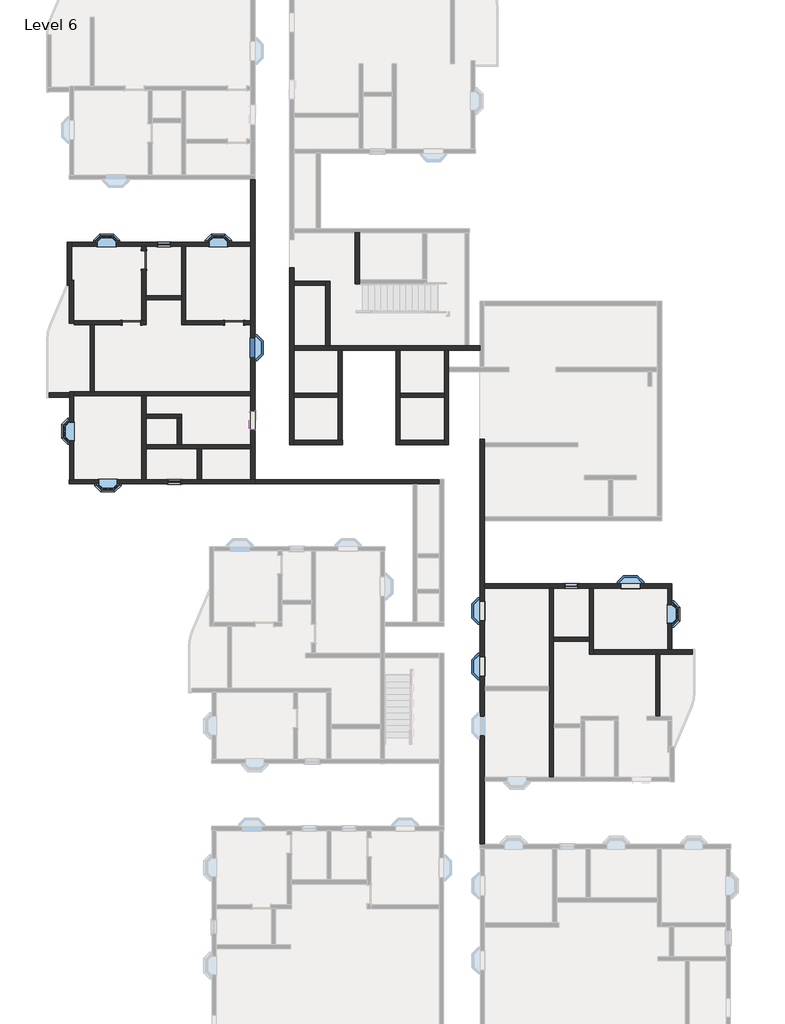
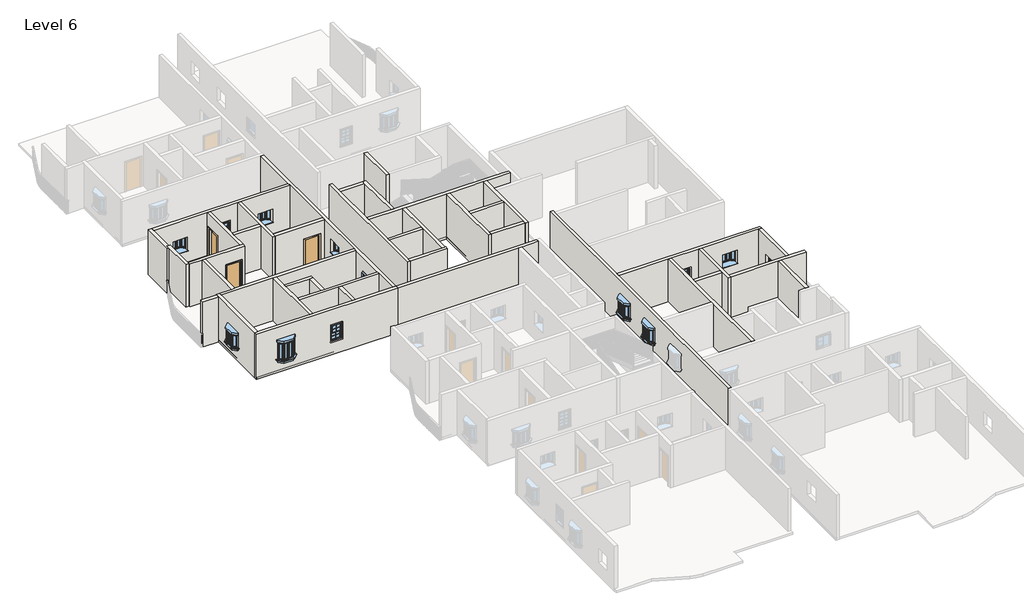
# One storey, part 3 of 14: 40 walls, 13 windows, 3 doors.
"""IFC4 building model written with IfcOpenShell, lengths in millimetres."""

from ifc_helpers import new_model, si_unit, frame, origin, place, context, project, spatial, polyline, outline, extrude, faceted_brep, transform, mapped, element, save
from components import door_54dd4da4, window_910x1210mm_154f9356, window_910x910mm_67ef725a, window_8debb0fa, windows_sgl_w_glazing_bars_910x910mm_256712d0

model = new_model("IFC4")

# Units and contexts
model_context = context("Model", 3, world=origin())
ifc_project = project(units=[si_unit("LENGTHUNIT", "METRE", prefix="MILLI")], contexts=[model_context])

# Site, building, storey
site = spatial("IfcSite", under=ifc_project)
building = spatial("IfcBuilding", under=site)
storey = spatial("IfcBuildingStorey", under=building, Name="Level 6", Elevation=15240.0)

# Doors
placement = place(None, origin())
door_shape = door_54dd4da4(model_context)
element("IfcDoor", 1, ObjectType="Single-Flush : 36\" x 84\"", at=placement, inside=storey, context=model_context, shape_type="MappedRepresentation", body=[
    mapped(door_shape, transform((-11210.3891351, 10605.7083494, 15240.0), x_axis=(1.0, 0.0, 0.0), y_axis=(0.0, 1.0, 0.0), z_axis=(0.0, 0.0, 1.0))),
])
element("IfcDoor", 2, ObjectType="Single-Flush : 36\" x 84\"", at=placement, inside=storey, context=model_context, shape_type="MappedRepresentation", body=[
    mapped(door_shape, transform((-15610.9391351, 13672.7583494, 15240.0), x_axis=(0.0, -1.0, 0.0), y_axis=(1.0, 0.0, 0.0), z_axis=(0.0, 0.0, 1.0))),
])
element("IfcDoor", 3, ObjectType="Single-Flush : 36\" x 84\"", at=placement, inside=storey, context=model_context, shape_type="MappedRepresentation", body=[
    mapped(door_shape, transform((-16220.5391351, 10605.7083494, 15240.0), x_axis=(1.0, 0.0, 0.0), y_axis=(0.0, 1.0, 0.0), z_axis=(0.0, 0.0, 1.0))),
])

# Walls
element("IfcWall", 4, ObjectType="4.5\" p", at=placement, inside=storey, context=model_context, shape_type="Brep", body=[
    faceted_brep([(-15509.3391351, 4456.3873146, 15240.0), (-13007.4391351, 4456.3873146, 15240.0), (-12804.2391351, 4456.3873146, 15240.0), (-10397.5891351, 4456.3873146, 15240.0), (-10397.5891351, 4456.3873146, 18288.0), (-12804.2391351, 4456.3873146, 18288.0), (-13007.4391351, 4456.3873146, 18288.0), (-15509.3391351, 4456.3873146, 18288.0), (-15509.3391351, 4659.5873146, 15240.0), (-15509.3391351, 4659.5873146, 18288.0), (-13985.3391351, 4659.5873146, 18288.0), (-13782.1391351, 4659.5873146, 18288.0), (-10397.5891351, 4659.5873146, 18288.0), (-10397.5891351, 4659.5873146, 15240.0), (-13782.1391351, 4659.5873146, 15240.0), (-13985.3391351, 4659.5873146, 15240.0)], [[[0, 1, 2, 3, 4, 5, 6, 7]], [[8, 9, 10, 11, 12, 13, 14, 15]], [[3, 2, 1, 0, 8, 15, 14, 13]], [[7, 6, 5, 4, 12, 11, 10, 9]], [[4, 3, 13, 12]], [[0, 7, 9, 8]]]),
])
element("IfcWall", 5, ObjectType="4.5\" p", at=placement, inside=storey, context=model_context, shape_type="SweptSolid", body=[
    extrude(outline(polyline([(-13007.4391351, 2953.9583494), (-13007.4391351, 4456.3873146), (-12804.2391351, 4456.3873146), (-12804.2391351, 2953.9583494), (-13007.4391351, 2953.9583494)])), frame((0.0, 0.0, 15240.0), z_axis=(0.0, 0.0, 1.0), x_axis=(1.0, 0.0, 0.0)), (0.0, 0.0, 1.0), 3048.0),
])
element("IfcWall", 6, ObjectType="4.5\" p", at=placement, inside=storey, context=model_context, shape_type="Brep", body=[
    faceted_brep([(-15509.3391351, 5953.2975261, 15240.0), (-13985.3391351, 5953.2975261, 15240.0), (-13782.1391351, 5953.2975261, 15240.0), (-13782.1391351, 5953.2975261, 18288.0), (-13985.3391351, 5953.2975261, 18288.0), (-15509.3391351, 5953.2975261, 18288.0), (-15509.3391351, 6156.4975261, 15240.0), (-15509.3391351, 6156.4975261, 18288.0), (-13782.1391351, 6156.4975261, 18288.0), (-13782.1391351, 6156.4975261, 15240.0)], [[[0, 1, 2, 3, 4, 5]], [[6, 7, 8, 9]], [[2, 1, 0, 6, 9]], [[5, 4, 3, 8, 7]], [[0, 5, 7, 6]], [[3, 2, 9, 8]]]),
])
element("IfcWall", 7, ObjectType="4.5\" p", at=placement, inside=storey, context=model_context, shape_type="SweptSolid", body=[
    extrude(outline(polyline([(-13985.3391351, 4659.5873146), (-13985.3391351, 5953.2975261), (-13782.1391351, 5953.2975261), (-13782.1391351, 4659.5873146), (-13985.3391351, 4659.5873146)])), frame((0.0, 0.0, 15240.0), z_axis=(0.0, 0.0, 1.0), x_axis=(1.0, 0.0, 0.0)), (0.0, 0.0, 1.0), 3048.0),
])
element("IfcWall", 8, ObjectType="4.5\" p", at=placement, inside=storey, context=model_context, shape_type="Brep", body=[
    faceted_brep([(-15712.5391351, 13215.5583494, 17373.6), (-15712.5391351, 13215.5583494, 15240.0), (-15712.5391351, 10707.3083494, 15240.0), (-15712.5391351, 10707.3083494, 18288.0), (-15712.5391351, 14333.1583494, 18288.0), (-15712.5391351, 14333.1583494, 15240.0), (-15712.5391351, 14129.9583494, 15240.0), (-15712.5391351, 14129.9583494, 17373.6), (-15509.3391351, 10707.3083494, 15240.0), (-15509.3391351, 11723.3083494, 15240.0), (-15509.3391351, 11926.5083494, 15240.0), (-15509.3391351, 13215.5583494, 15240.0), (-15509.3391351, 13215.5583494, 17373.6), (-15509.3391351, 14129.9583494, 17373.6), (-15509.3391351, 14129.9583494, 15240.0), (-15509.3391351, 14333.1583494, 15240.0), (-15509.3391351, 14333.1583494, 18288.0), (-15509.3391351, 11926.5083494, 18288.0), (-15509.3391351, 11723.3083494, 18288.0), (-15509.3391351, 10707.3083494, 18288.0)], [[[0, 1, 2, 3, 4, 5, 6, 7]], [[8, 9, 10, 11, 12, 13, 14, 15, 16, 17, 18, 19]], [[6, 5, 15, 14]], [[2, 1, 11, 10, 9, 8]], [[4, 3, 19, 18, 17, 16]], [[3, 2, 8, 19]], [[5, 4, 16, 15]], [[12, 11, 1, 0]], [[13, 12, 0, 7]], [[14, 13, 7, 6]]]),
])
element("IfcWall", 9, ObjectType="4.5\" p", at=placement, inside=storey, context=model_context, shape_type="Brep", body=[
    faceted_brep([(-13769.4391351, 14333.1583494, 15240.0), (-13769.4391351, 11926.5083494, 15240.0), (-13769.4391351, 11723.3083494, 15240.0), (-13769.4391351, 10504.1083494, 15240.0), (-13769.4391351, 10504.1083494, 18288.0), (-13769.4391351, 11723.3083494, 18288.0), (-13769.4391351, 11926.5083494, 18288.0), (-13769.4391351, 14333.1583494, 18288.0), (-13566.2391351, 14333.1583494, 15240.0), (-13566.2391351, 14333.1583494, 18288.0), (-13566.2391351, 10707.3083494, 18288.0), (-13566.2391351, 10504.1083494, 18288.0), (-13566.2391351, 10504.1083494, 15240.0), (-13566.2391351, 10707.3083494, 15240.0)], [[[0, 1, 2, 3, 4, 5, 6, 7]], [[8, 9, 10, 11, 12, 13]], [[3, 2, 1, 0, 8, 13, 12]], [[7, 6, 5, 4, 11, 10, 9]], [[0, 7, 9, 8]], [[4, 3, 12, 11]]]),
])
element("IfcWall", 10, ObjectType="4.5\" p", at=placement, inside=storey, context=model_context, shape_type="SweptSolid", body=[
    extrude(outline(polyline([(17373.6, -10753.1891351), (15240.0, -10753.1891351), (15240.0, -10397.5891351), (18288.0, -10397.5891351), (18288.0, -13566.2391351), (15240.0, -13566.2391351), (15240.0, -11667.5891351), (17373.6, -11667.5891351), (17373.6, -10753.1891351)])), frame((0.0, 10504.1083494, 0.0), z_axis=(0.0, 1.0, 0.0), x_axis=(0.0, 0.0, 1.0)), (0.0, 0.0, 1.0), 203.2),
])
element("IfcWall", 11, ObjectType="4.5\" p", at=placement, inside=storey, context=model_context, shape_type="SweptSolid", body=[
    extrude(outline(polyline([(-13769.4391351, 11723.3083494), (-15509.3391351, 11723.3083494), (-15509.3391351, 11926.5083494), (-13769.4391351, 11926.5083494), (-13769.4391351, 11723.3083494)])), frame((0.0, 0.0, 15240.0), z_axis=(0.0, 0.0, 1.0), x_axis=(1.0, 0.0, 0.0)), (0.0, 0.0, 1.0), 3048.0),
])
element("IfcWall", 12, ObjectType="4.5\" p", at=placement, inside=storey, context=model_context, shape_type="SweptSolid", body=[
    extrude(outline(polyline([(-6739.9891351, 12429.8715905), (-8289.3891351, 12429.8715905), (-8289.3891351, 12633.0715905), (-6739.9891351, 12633.0715905), (-6739.9891351, 12429.8715905)])), frame((0.0, 0.0, 15240.0), z_axis=(0.0, 0.0, 1.0), x_axis=(1.0, 0.0, 0.0)), (0.0, 0.0, 1.0), 3048.0),
])
element("IfcWall", 13, ObjectType="4.5\" p", at=placement, inside=storey, context=model_context, shape_type="SweptSolid", body=[
    extrude(outline(polyline([(-6130.3891351, 6970.2449943), (-8289.3891351, 6970.2449943), (-8289.3891351, 7173.4449943), (-6130.3891351, 7173.4449943), (-6130.3891351, 6970.2449943)])), frame((0.0, 0.0, 15240.0), z_axis=(0.0, 0.0, 1.0), x_axis=(1.0, 0.0, 0.0)), (0.0, 0.0, 1.0), 3048.0),
])
element("IfcWall", 14, ObjectType="4.5\" p", at=placement, inside=storey, context=model_context, shape_type="SweptSolid", body=[
    extrude(outline(polyline([(-948.7891351, 6970.2449943), (-3107.7891351, 6970.2449943), (-3107.7891351, 7173.4449943), (-948.7891351, 7173.4449943), (-948.7891351, 6970.2449943)])), frame((0.0, 0.0, 15240.0), z_axis=(0.0, 0.0, 1.0), x_axis=(1.0, 0.0, 0.0)), (0.0, 0.0, 1.0), 3048.0),
])
element("IfcWall", 15, ObjectType="4.5\" p", at=placement, inside=storey, context=model_context, shape_type="Brep", body=[
    faceted_brep([(-5298.5391351, 14988.9215905, 15240.0), (-5298.5391351, 12506.0715905, 15240.0), (-5298.5391351, 12506.0715905, 18288.0), (-5298.5391351, 14988.9215905, 18288.0), (-5095.3391351, 14988.9215905, 15240.0), (-5095.3391351, 14988.9215905, 18288.0), (-5095.3391351, 12709.2715905, 18288.0), (-5095.3391351, 12506.0715905, 18288.0), (-5095.3391351, 12506.0715905, 15240.0), (-5095.3391351, 12709.2715905, 15240.0)], [[[0, 1, 2, 3]], [[4, 5, 6, 7, 8, 9]], [[1, 0, 4, 9, 8]], [[3, 2, 7, 6, 5]], [[0, 3, 5, 4]], [[2, 1, 8, 7]]]),
])
element("IfcWall", 16, ObjectType="4.5\" p", at=placement, inside=storey, context=model_context, shape_type="SweptSolid", body=[
    extrude(outline(polyline([(-948.7891351, 4665.1949943), (-3107.7891351, 4665.1949943), (-3107.7891351, 4868.3949943), (-948.7891351, 4868.3949943), (-948.7891351, 4665.1949943)])), frame((0.0, 0.0, 15240.0), z_axis=(0.0, 0.0, 1.0), x_axis=(1.0, 0.0, 0.0)), (0.0, 0.0, 1.0), 3048.0),
])
element("IfcWall", 17, ObjectType="4.5\" p", at=placement, inside=storey, context=model_context, shape_type="Brep", body=[
    faceted_brep([(4184.4880523, -2336.4042694, 15240.0), (4184.4880523, -7130.6542694, 15240.0), (4184.4880523, -7333.8542694, 15240.0), (4184.4880523, -11556.6042694, 15240.0), (4184.4880523, -11556.6042694, 18288.0), (4184.4880523, -7333.8542694, 18288.0), (4184.4880523, -7130.6542694, 18288.0), (4184.4880523, -2336.4042694, 18288.0), (4387.6880523, -2336.4042694, 15240.0), (4387.6880523, -2336.4042694, 18288.0), (4387.6880523, -4736.7042694, 18288.0), (4387.6880523, -4939.9042694, 18288.0), (4387.6880523, -8959.4542694, 18288.0), (4387.6880523, -9162.6542694, 18288.0), (4387.6880523, -11556.6042694, 18288.0), (4387.6880523, -11556.6042694, 15240.0), (4387.6880523, -9162.6542694, 15240.0), (4387.6880523, -8959.4542694, 15240.0), (4387.6880523, -4939.9042694, 15240.0), (4387.6880523, -4736.7042694, 15240.0)], [[[0, 1, 2, 3, 4, 5, 6, 7]], [[8, 9, 10, 11, 12, 13, 14, 15, 16, 17, 18, 19]], [[3, 2, 1, 0, 8, 19, 18, 17, 16, 15]], [[7, 6, 5, 4, 14, 13, 12, 11, 10, 9]], [[4, 3, 15, 14]], [[0, 7, 9, 8]]]),
])
element("IfcWall", 18, ObjectType="4.5\" p", at=placement, inside=storey, context=model_context, shape_type="Brep", body=[
    faceted_brep([(803.8108649, 4915.2957306, 15240.0), (803.8108649, -14845.9042694, 15240.0), (803.8108649, -14845.9042694, 18288.0), (803.8108649, 4915.2957306, 18288.0), (803.8108649, -9516.0542694, 17350.0), (803.8108649, -9516.0542694, 16440.0), (803.8108649, -8606.0542694, 16440.0), (803.8108649, -8606.0542694, 17350.0), (803.8108649, -3909.0042694, 17350.0), (803.8108649, -3909.0042694, 16440.0), (803.8108649, -2999.0042694, 16440.0), (803.8108649, -2999.0042694, 17350.0), (803.8108649, -6620.4542694, 17350.0), (803.8108649, -6620.4542694, 16440.0), (803.8108649, -5710.4542694, 16440.0), (803.8108649, -5710.4542694, 17350.0), (1007.0108649, 4915.2957306, 15240.0), (1007.0108649, 4915.2957306, 18288.0), (1007.0108649, 4754.0949943, 18288.0), (1007.0108649, 4550.8949943, 18288.0), (1007.0108649, 1143.3957306, 18288.0), (1007.0108649, 940.1957306, 18288.0), (1007.0108649, -2133.2042694, 18288.0), (1007.0108649, -2336.4042694, 18288.0), (1007.0108649, -7130.6542694, 18288.0), (1007.0108649, -7333.8542694, 18288.0), (1007.0108649, -11556.6042694, 18288.0), (1007.0108649, -11759.8042694, 18288.0), (1007.0108649, -14845.9042694, 18288.0), (1007.0108649, -14845.9042694, 15240.0), (1007.0108649, -11759.8042694, 15240.0), (1007.0108649, -11556.6042694, 15240.0), (1007.0108649, -7333.8542694, 15240.0), (1007.0108649, -7130.6542694, 15240.0), (1007.0108649, -2336.4042694, 15240.0), (1007.0108649, -2133.2042694, 15240.0), (1007.0108649, 940.1957306, 15240.0), (1007.0108649, 1143.3957306, 15240.0), (1007.0108649, 4550.8949943, 15240.0), (1007.0108649, 4754.0949943, 15240.0), (1007.0108649, -9516.0542694, 17350.0), (1007.0108649, -8606.0542694, 17350.0), (1007.0108649, -8606.0542694, 16440.0), (1007.0108649, -9516.0542694, 16440.0), (1007.0108649, -3909.0042694, 17350.0), (1007.0108649, -2999.0042694, 17350.0), (1007.0108649, -2999.0042694, 16440.0), (1007.0108649, -3909.0042694, 16440.0), (1007.0108649, -6620.4542694, 17350.0), (1007.0108649, -5710.4542694, 17350.0), (1007.0108649, -5710.4542694, 16440.0), (1007.0108649, -6620.4542694, 16440.0)], [[[0, 1, 2, 3], [4, 5, 6, 7], [8, 9, 10, 11], [12, 13, 14, 15]], [[16, 17, 18, 19, 20, 21, 22, 23, 24, 25, 26, 27, 28, 29, 30, 31, 32, 33, 34, 35, 36, 37, 38, 39], [40, 41, 42, 43], [44, 45, 46, 47], [48, 49, 50, 51]], [[1, 0, 16, 39, 38, 37, 36, 35, 34, 33, 32, 31, 30, 29]], [[3, 2, 28, 27, 26, 25, 24, 23, 22, 21, 20, 19, 18, 17]], [[0, 3, 17, 16]], [[2, 1, 29, 28]], [[5, 4, 40, 43]], [[6, 5, 43, 42]], [[7, 6, 42, 41]], [[4, 7, 41, 40]], [[9, 8, 44, 47]], [[10, 9, 47, 46]], [[11, 10, 46, 45]], [[8, 11, 45, 44]], [[13, 12, 48, 51]], [[14, 13, 51, 50]], [[15, 14, 50, 49]], [[12, 15, 49, 48]]]),
])
element("IfcWall", 19, ObjectType="4.5\" p", at=placement, inside=storey, context=model_context, shape_type="SweptSolid", body=[
    extrude(outline(polyline([(6127.5880523, -4939.9042694), (4387.6880523, -4939.9042694), (4387.6880523, -4736.7042694), (6127.5880523, -4736.7042694), (6127.5880523, -4939.9042694)])), frame((0.0, 0.0, 15240.0), z_axis=(0.0, 0.0, 1.0), x_axis=(1.0, 0.0, 0.0)), (0.0, 0.0, 1.0), 3048.0),
])
element("IfcWall", 20, ObjectType="4.5\" p", at=placement, inside=storey, context=model_context, shape_type="Brep", body=[
    faceted_brep([(6127.5880523, -2336.4042694, 15240.0), (6127.5880523, -4736.7042694, 15240.0), (6127.5880523, -4939.9042694, 15240.0), (6127.5880523, -5555.8542694, 15240.0), (6127.5880523, -5555.8542694, 18288.0), (6127.5880523, -4939.9042694, 18288.0), (6127.5880523, -4736.7042694, 18288.0), (6127.5880523, -2336.4042694, 18288.0), (6330.7880523, -2336.4042694, 15240.0), (6330.7880523, -2336.4042694, 18288.0), (6330.7880523, -5352.6542694, 18288.0), (6330.7880523, -5555.8542694, 18288.0), (6330.7880523, -5555.8542694, 15240.0), (6330.7880523, -5352.6542694, 15240.0)], [[[0, 1, 2, 3, 4, 5, 6, 7]], [[8, 9, 10, 11, 12, 13]], [[3, 2, 1, 0, 8, 13, 12]], [[7, 6, 5, 4, 11, 10, 9]], [[0, 7, 9, 8]], [[4, 3, 12, 11]]]),
])
element("IfcWall", 21, ObjectType="4.5\" p", at=placement, inside=storey, context=model_context, shape_type="Brep", body=[
    faceted_brep([(6330.7880523, -5555.8542694, 15240.0), (9371.2322031, -5555.8542694, 15240.0), (9574.4322031, -5555.8542694, 15240.0), (11163.1380523, -5555.8542694, 15240.0), (11163.1380523, -5555.8542694, 18288.0), (9574.4322031, -5555.8542694, 18288.0), (9371.2322031, -5555.8542694, 18288.0), (6330.7880523, -5555.8542694, 18288.0), (6330.7880523, -5352.6542694, 15240.0), (6330.7880523, -5352.6542694, 18288.0), (9956.6380523, -5352.6542694, 18288.0), (10159.8380523, -5352.6542694, 18288.0), (11163.1380523, -5352.6542694, 18288.0), (11163.1380523, -5352.6542694, 15240.0), (10159.8380523, -5352.6542694, 15240.0), (9956.6380523, -5352.6542694, 15240.0)], [[[0, 1, 2, 3, 4, 5, 6, 7]], [[8, 9, 10, 11, 12, 13, 14, 15]], [[3, 2, 1, 0, 8, 15, 14, 13]], [[4, 3, 13, 12]], [[7, 6, 5, 4, 12, 11, 10, 9]], [[0, 7, 9, 8]]]),
])
element("IfcWall", 22, ObjectType="4.5\" p", at=placement, inside=storey, context=model_context, shape_type="SweptSolid", body=[
    extrude(outline(polyline([(9371.2322031, -8578.4542694), (9371.2322031, -5555.8542694), (9574.4322031, -5555.8542694), (9574.4322031, -8578.4542694), (9371.2322031, -8578.4542694)])), frame((0.0, 0.0, 15240.0), z_axis=(0.0, 0.0, 1.0), x_axis=(1.0, 0.0, 0.0)), (0.0, 0.0, 1.0), 3048.0),
])
element("IfcWall", 23, ObjectType="9\"", at=placement, inside=storey, context=model_context, shape_type="Brep", body=[
    faceted_brep([(-10181.6891351, 2953.9583494, 15240.0), (-10194.3891351, 2953.9583494, 15240.0), (-10397.5891351, 2953.9583494, 15240.0), (-12804.2391351, 2953.9583494, 15240.0), (-13007.4391351, 2953.9583494, 15240.0), (-15509.3391351, 2953.9583494, 15240.0), (-15712.5391351, 2953.9583494, 15240.0), (-19033.5891351, 2953.9583494, 15240.0), (-19236.7891351, 2953.9583494, 15240.0), (-19249.4891351, 2953.9583494, 15240.0), (-19249.4891351, 2953.9583494, 18288.0), (-19236.7891351, 2953.9583494, 18288.0), (-19033.5891351, 2953.9583494, 18288.0), (-15712.5391351, 2953.9583494, 18288.0), (-15509.3391351, 2953.9583494, 18288.0), (-13007.4391351, 2953.9583494, 18288.0), (-12804.2391351, 2953.9583494, 18288.0), (-10397.5891351, 2953.9583494, 18288.0), (-10194.3891351, 2953.9583494, 18288.0), (-10181.6891351, 2953.9583494, 18288.0), (-13794.8391351, 2953.9583494, 17221.2), (-14455.2391351, 2953.9583494, 17221.2), (-14455.2391351, 2953.9583494, 16154.4), (-13794.8391351, 2953.9583494, 16154.4), (-16918.0641351, 2953.9583494, 17350.0), (-17828.0641351, 2953.9583494, 17350.0), (-17828.0641351, 2953.9583494, 16140.0), (-16918.0641351, 2953.9583494, 16140.0), (-10181.6891351, 2750.7583494, 15240.0), (-10181.6891351, 2750.7583494, 18288.0), (-19249.4891351, 2750.7583494, 18288.0), (-19249.4891351, 2750.7583494, 15240.0), (-13794.8391351, 2750.7583494, 17221.2), (-13794.8391351, 2750.7583494, 16154.4), (-14455.2391351, 2750.7583494, 16154.4), (-14455.2391351, 2750.7583494, 17221.2), (-16918.0641351, 2750.7583494, 17350.0), (-16918.0641351, 2750.7583494, 16140.0), (-17828.0641351, 2750.7583494, 16140.0), (-17828.0641351, 2750.7583494, 17350.0)], [[[0, 1, 2, 3, 4, 5, 6, 7, 8, 9, 10, 11, 12, 13, 14, 15, 16, 17, 18, 19], [20, 21, 22, 23], [24, 25, 26, 27]], [[28, 29, 30, 31], [32, 33, 34, 35], [36, 37, 38, 39]], [[9, 8, 7, 6, 5, 4, 3, 2, 1, 0, 28, 31]], [[10, 9, 31, 30]], [[19, 18, 17, 16, 15, 14, 13, 12, 11, 10, 30, 29]], [[0, 19, 29, 28]], [[33, 32, 20, 23]], [[34, 33, 23, 22]], [[35, 34, 22, 21]], [[32, 35, 21, 20]], [[37, 36, 24, 27]], [[38, 37, 27, 26]], [[39, 38, 26, 25]], [[36, 39, 25, 24]]]),
])
element("IfcWall", 24, ObjectType="9\"", at=placement, inside=storey, context=model_context, shape_type="Brep", body=[
    faceted_brep([(-19033.5891351, 2953.9583494, 15240.0), (-19033.5891351, 7037.0083494, 15240.0), (-19033.5891351, 7240.2083494, 15240.0), (-19033.5891351, 7240.2083494, 18288.0), (-19033.5891351, 7037.0083494, 18288.0), (-19033.5891351, 2953.9583494, 18288.0), (-19033.5891351, 4854.8083494, 17064.4), (-19033.5891351, 5764.8083494, 17064.4), (-19033.5891351, 5764.8083494, 16154.4), (-19033.5891351, 4854.8083494, 16154.4), (-19236.7891351, 2953.9583494, 15240.0), (-19236.7891351, 2953.9583494, 18288.0), (-19236.7891351, 7240.2083494, 18288.0), (-19236.7891351, 7240.2083494, 15240.0), (-19236.7891351, 4854.8083494, 17064.4), (-19236.7891351, 4854.8083494, 16154.4), (-19236.7891351, 5764.8083494, 16154.4), (-19236.7891351, 5764.8083494, 17064.4)], [[[0, 1, 2, 3, 4, 5], [6, 7, 8, 9]], [[10, 11, 12, 13], [14, 15, 16, 17]], [[2, 1, 0, 10, 13]], [[5, 4, 3, 12, 11]], [[0, 5, 11, 10]], [[3, 2, 13, 12]], [[15, 14, 6, 9]], [[16, 15, 9, 8]], [[17, 16, 8, 7]], [[14, 17, 7, 6]]]),
])
element("IfcWall", 25, ObjectType="9\"", at=placement, inside=storey, context=model_context, shape_type="Brep", body=[
    faceted_brep([(-10194.3891351, 2953.9583494, 15240.0), (-10194.3891351, 17597.0583494, 15240.0), (-10194.3891351, 17597.0583494, 18288.0), (-10194.3891351, 2953.9583494, 18288.0), (-10194.3891351, 9841.5083494, 17350.0), (-10194.3891351, 9841.5083494, 16440.0), (-10194.3891351, 8931.5083494, 16440.0), (-10194.3891351, 8931.5083494, 17350.0), (-10194.3891351, 5393.297832, 17350.0), (-10194.3891351, 6303.297832, 17350.0), (-10194.3891351, 6303.297832, 16440.0), (-10194.3891351, 5393.297832, 16440.0), (-10397.5891351, 2953.9583494, 15240.0), (-10397.5891351, 2953.9583494, 18288.0), (-10397.5891351, 4456.3873146, 18288.0), (-10397.5891351, 4659.5873146, 18288.0), (-10397.5891351, 7037.0083494, 18288.0), (-10397.5891351, 7240.2083494, 18288.0), (-10397.5891351, 10504.1083494, 18288.0), (-10397.5891351, 10707.3083494, 18288.0), (-10397.5891351, 14333.1583494, 18288.0), (-10397.5891351, 14536.3583494, 18288.0), (-10397.5891351, 17597.0583494, 18288.0), (-10397.5891351, 17597.0583494, 15240.0), (-10397.5891351, 14536.3583494, 15240.0), (-10397.5891351, 14333.1583494, 15240.0), (-10397.5891351, 10707.3083494, 15240.0), (-10397.5891351, 10504.1083494, 15240.0), (-10397.5891351, 7240.2083494, 15240.0), (-10397.5891351, 7037.0083494, 15240.0), (-10397.5891351, 4659.5873146, 15240.0), (-10397.5891351, 4456.3873146, 15240.0), (-10397.5891351, 9841.5083494, 17350.0), (-10397.5891351, 8931.5083494, 17350.0), (-10397.5891351, 8931.5083494, 16440.0), (-10397.5891351, 9841.5083494, 16440.0), (-10397.5891351, 5393.297832, 17350.0), (-10397.5891351, 5393.297832, 16440.0), (-10397.5891351, 6303.297832, 16440.0), (-10397.5891351, 6303.297832, 17350.0)], [[[0, 1, 2, 3], [4, 5, 6, 7], [8, 9, 10, 11]], [[12, 13, 14, 15, 16, 17, 18, 19, 20, 21, 22, 23, 24, 25, 26, 27, 28, 29, 30, 31], [32, 33, 34, 35], [36, 37, 38, 39]], [[1, 0, 12, 31, 30, 29, 28, 27, 26, 25, 24, 23]], [[2, 1, 23, 22]], [[3, 2, 22, 21, 20, 19, 18, 17, 16, 15, 14, 13]], [[0, 3, 13, 12]], [[5, 4, 32, 35]], [[6, 5, 35, 34]], [[7, 6, 34, 33]], [[4, 7, 33, 32]], [[37, 36, 8, 11]], [[38, 37, 11, 10]], [[39, 38, 10, 9]], [[36, 39, 9, 8]]]),
])
element("IfcWall", 26, ObjectType="9\"", at=placement, inside=storey, context=model_context, shape_type="SweptSolid", body=[
    extrude(outline(polyline([(-19249.4891351, 6979.8583494), (-20240.0891351, 6979.8583494), (-20240.0891351, 7183.0583494), (-19249.4891351, 7183.0583494), (-19249.4891351, 6979.8583494)])), frame((0.0, 0.0, 15240.0), z_axis=(0.0, 0.0, 1.0), x_axis=(1.0, 0.0, 0.0)), (0.0, 0.0, 1.0), 3048.0),
])
element("IfcWall", 27, ObjectType="9\"", at=placement, inside=storey, context=model_context, shape_type="Brep", body=[
    faceted_brep([(-19147.8891351, 12435.1858981, 15240.0), (-19147.8891351, 14333.1583494, 15240.0), (-19147.8891351, 14536.3583494, 15240.0), (-19147.8891351, 14549.0583494, 15240.0), (-19147.8891351, 14549.0583494, 18288.0), (-19147.8891351, 14536.3583494, 18288.0), (-19147.8891351, 14333.1583494, 18288.0), (-19147.8891351, 12435.1858981, 18288.0), (-19351.0891351, 12435.1858981, 15240.0), (-19351.0891351, 12435.1858981, 18288.0), (-19351.0891351, 14549.0583494, 18288.0), (-19351.0891351, 14549.0583494, 15240.0)], [[[0, 1, 2, 3, 4, 5, 6, 7]], [[8, 9, 10, 11]], [[3, 2, 1, 0, 8, 11]], [[4, 3, 11, 10]], [[7, 6, 5, 4, 10, 9]], [[0, 7, 9, 8]]]),
])
element("IfcWall", 28, ObjectType="9\"", at=placement, inside=storey, context=model_context, shape_type="Brep", body=[
    faceted_brep([(-19147.8891351, 14333.1583494, 15240.0), (-15712.5391351, 14333.1583494, 15240.0), (-15509.3391351, 14333.1583494, 15240.0), (-13769.4391351, 14333.1583494, 15240.0), (-13566.2391351, 14333.1583494, 15240.0), (-10397.5891351, 14333.1583494, 15240.0), (-10397.5891351, 14333.1583494, 18288.0), (-13566.2391351, 14333.1583494, 18288.0), (-13769.4391351, 14333.1583494, 18288.0), (-15509.3391351, 14333.1583494, 18288.0), (-15712.5391351, 14333.1583494, 18288.0), (-19147.8891351, 14333.1583494, 18288.0), (-17885.2141351, 14333.1583494, 17064.4), (-16975.2141351, 14333.1583494, 17064.4), (-16975.2141351, 14333.1583494, 16154.4), (-17885.2141351, 14333.1583494, 16154.4), (-12436.9141351, 14333.1583494, 17064.4), (-11526.9141351, 14333.1583494, 17064.4), (-11526.9141351, 14333.1583494, 16154.4), (-12436.9141351, 14333.1583494, 16154.4), (-14309.1891351, 14333.1583494, 17221.2), (-14309.1891351, 14333.1583494, 16154.4), (-14969.5891351, 14333.1583494, 16154.4), (-14969.5891351, 14333.1583494, 17221.2), (-19147.8891351, 14536.3583494, 15240.0), (-19147.8891351, 14536.3583494, 18288.0), (-10397.5891351, 14536.3583494, 18288.0), (-10397.5891351, 14536.3583494, 15240.0), (-17885.2141351, 14536.3583494, 17064.4), (-17885.2141351, 14536.3583494, 16154.4), (-16975.2141351, 14536.3583494, 16154.4), (-16975.2141351, 14536.3583494, 17064.4), (-12436.9141351, 14536.3583494, 17064.4), (-12436.9141351, 14536.3583494, 16154.4), (-11526.9141351, 14536.3583494, 16154.4), (-11526.9141351, 14536.3583494, 17064.4), (-14309.1891351, 14536.3583494, 17221.2), (-14969.5891351, 14536.3583494, 17221.2), (-14969.5891351, 14536.3583494, 16154.4), (-14309.1891351, 14536.3583494, 16154.4)], [[[0, 1, 2, 3, 4, 5, 6, 7, 8, 9, 10, 11], [12, 13, 14, 15], [16, 17, 18, 19], [20, 21, 22, 23]], [[24, 25, 26, 27], [28, 29, 30, 31], [32, 33, 34, 35], [36, 37, 38, 39]], [[5, 4, 3, 2, 1, 0, 24, 27]], [[11, 10, 9, 8, 7, 6, 26, 25]], [[6, 5, 27, 26]], [[0, 11, 25, 24]], [[29, 28, 12, 15]], [[30, 29, 15, 14]], [[31, 30, 14, 13]], [[28, 31, 13, 12]], [[33, 32, 16, 19]], [[34, 33, 19, 18]], [[35, 34, 18, 17]], [[32, 35, 17, 16]], [[21, 20, 36, 39]], [[22, 21, 39, 38]], [[23, 22, 38, 37]], [[20, 23, 37, 36]]]),
])
element("IfcWall", 29, ObjectType="9\"", at=placement, inside=storey, context=model_context, shape_type="SweptSolid", body=[
    extrude(outline(polyline([(-19249.4891351, 10585.5474528), (-19249.4891351, 12672.4473407), (-19046.2891351, 12672.4473407), (-19046.2891351, 10585.5474528), (-19249.4891351, 10585.5474528)])), frame((0.0, 0.0, 15240.0), z_axis=(0.0, 0.0, 1.0), x_axis=(1.0, 0.0, 0.0)), (0.0, 0.0, 1.0), 3048.0),
])
element("IfcWall", 30, ObjectType="9\" w", at=placement, inside=storey, context=model_context, shape_type="Brep", body=[
    faceted_brep([(-1177.3891351, 2953.9583494, 15240.0), (-10181.6891351, 2953.9583494, 15240.0), (-10181.6891351, 2953.9583494, 18288.0), (-1177.3891351, 2953.9583494, 18288.0), (-1177.3891351, 2750.7583494, 15240.0), (-1177.3891351, 2750.7583494, 18288.0), (-2269.5891351, 2750.7583494, 18288.0), (-2472.7891351, 2750.7583494, 18288.0), (-10181.6891351, 2750.7583494, 18288.0), (-10181.6891351, 2750.7583494, 15240.0), (-2472.7891351, 2750.7583494, 15240.0), (-2269.5891351, 2750.7583494, 15240.0)], [[[0, 1, 2, 3]], [[4, 5, 6, 7, 8, 9, 10, 11]], [[1, 0, 4, 11, 10, 9]], [[2, 1, 9, 8]], [[3, 2, 8, 7, 6, 5]], [[0, 3, 5, 4]]]),
])
element("IfcWall", 31, ObjectType="9\" w", at=placement, inside=storey, context=model_context, shape_type="Brep", body=[
    faceted_brep([(-15763.3391351, 10504.1083494, 17373.6), (-15763.3391351, 10504.1083494, 15240.0), (-15509.3391351, 10504.1083494, 15240.0), (-15509.3391351, 10504.1083494, 18288.0), (-18042.9891351, 10504.1083494, 18288.0), (-18246.1891351, 10504.1083494, 18288.0), (-19027.2391351, 10504.1083494, 18288.0), (-19027.2391351, 10504.1083494, 15240.0), (-18246.1891351, 10504.1083494, 15240.0), (-18042.9891351, 10504.1083494, 15240.0), (-16677.7391351, 10504.1083494, 15240.0), (-16677.7391351, 10504.1083494, 17373.6), (-15509.3391351, 10707.3083494, 15240.0), (-15712.5391351, 10707.3083494, 15240.0), (-15763.3391351, 10707.3083494, 15240.0), (-15763.3391351, 10707.3083494, 17373.6), (-16677.7391351, 10707.3083494, 17373.6), (-16677.7391351, 10707.3083494, 15240.0), (-19027.2391351, 10707.3083494, 15240.0), (-19027.2391351, 10707.3083494, 18288.0), (-15712.5391351, 10707.3083494, 18288.0), (-15509.3391351, 10707.3083494, 18288.0)], [[[0, 1, 2, 3, 4, 5, 6, 7, 8, 9, 10, 11]], [[12, 13, 14, 15, 16, 17, 18, 19, 20, 21]], [[2, 1, 14, 13, 12]], [[10, 9, 8, 7, 18, 17]], [[6, 5, 4, 3, 21, 20, 19]], [[7, 6, 19, 18]], [[3, 2, 12, 21]], [[15, 14, 1, 0]], [[16, 15, 0, 11]], [[17, 16, 11, 10]]]),
])
element("IfcWall", 32, ObjectType="9\" w", at=placement, inside=storey, context=model_context, shape_type="SweptSolid", body=[
    extrude(outline(polyline([(-18246.1891351, 7240.2083494), (-18246.1891351, 10504.1083494), (-18042.9891351, 10504.1083494), (-18042.9891351, 7240.2083494), (-18246.1891351, 7240.2083494)])), frame((0.0, 0.0, 15240.0), z_axis=(0.0, 0.0, 1.0), x_axis=(1.0, 0.0, 0.0)), (0.0, 0.0, 1.0), 3048.0),
])
element("IfcWall", 33, ObjectType="9\" w", at=placement, inside=storey, context=model_context, shape_type="Brep", body=[
    faceted_brep([(-19033.5891351, 7037.0083494, 15240.0), (-15712.5391351, 7037.0083494, 15240.0), (-15509.3391351, 7037.0083494, 15240.0), (-10397.5891351, 7037.0083494, 15240.0), (-10397.5891351, 7037.0083494, 18288.0), (-15509.3391351, 7037.0083494, 18288.0), (-15712.5391351, 7037.0083494, 18288.0), (-19033.5891351, 7037.0083494, 18288.0), (-19033.5891351, 7240.2083494, 15240.0), (-19033.5891351, 7240.2083494, 18288.0), (-18246.1891351, 7240.2083494, 18288.0), (-18042.9891351, 7240.2083494, 18288.0), (-10397.5891351, 7240.2083494, 18288.0), (-10397.5891351, 7240.2083494, 15240.0), (-18042.9891351, 7240.2083494, 15240.0), (-18246.1891351, 7240.2083494, 15240.0)], [[[0, 1, 2, 3, 4, 5, 6, 7]], [[8, 9, 10, 11, 12, 13, 14, 15]], [[3, 2, 1, 0, 8, 15, 14, 13]], [[7, 6, 5, 4, 12, 11, 10, 9]], [[0, 7, 9, 8]], [[4, 3, 13, 12]]]),
])
element("IfcWall", 34, ObjectType="9\" w", at=placement, inside=storey, context=model_context, shape_type="Brep", body=[
    faceted_brep([(-15712.5391351, 7037.0083494, 15240.0), (-15712.5391351, 2953.9583494, 15240.0), (-15712.5391351, 2953.9583494, 18288.0), (-15712.5391351, 7037.0083494, 18288.0), (-15509.3391351, 7037.0083494, 15240.0), (-15509.3391351, 7037.0083494, 18288.0), (-15509.3391351, 6156.4975261, 18288.0), (-15509.3391351, 5953.2975261, 18288.0), (-15509.3391351, 4659.5873146, 18288.0), (-15509.3391351, 4456.3873146, 18288.0), (-15509.3391351, 2953.9583494, 18288.0), (-15509.3391351, 2953.9583494, 15240.0), (-15509.3391351, 4456.3873146, 15240.0), (-15509.3391351, 4659.5873146, 15240.0), (-15509.3391351, 5953.2975261, 15240.0), (-15509.3391351, 6156.4975261, 15240.0)], [[[0, 1, 2, 3]], [[4, 5, 6, 7, 8, 9, 10, 11, 12, 13, 14, 15]], [[1, 0, 4, 15, 14, 13, 12, 11]], [[3, 2, 10, 9, 8, 7, 6, 5]], [[2, 1, 11, 10]], [[0, 3, 5, 4]]]),
])
element("IfcWall", 35, ObjectType="9\" w", at=placement, inside=storey, context=model_context, shape_type="Brep", body=[
    faceted_brep([(-8492.5891351, 13295.1410318, 15240.0), (-8492.5891351, 4652.4949943, 15240.0), (-8492.5891351, 4652.4949943, 18288.0), (-8492.5891351, 13295.1410318, 18288.0), (-8289.3891351, 13295.1410318, 15240.0), (-8289.3891351, 13295.1410318, 18288.0), (-8289.3891351, 12633.0715905, 18288.0), (-8289.3891351, 12429.8715905, 18288.0), (-8289.3891351, 9478.4949943, 18288.0), (-8289.3891351, 9275.2949943, 18288.0), (-8289.3891351, 7173.4449943, 18288.0), (-8289.3891351, 6970.2449943, 18288.0), (-8289.3891351, 4868.3949943, 18288.0), (-8289.3891351, 4665.1949943, 18288.0), (-8289.3891351, 4652.4949943, 18288.0), (-8289.3891351, 4652.4949943, 15240.0), (-8289.3891351, 4665.1949943, 15240.0), (-8289.3891351, 4868.3949943, 15240.0), (-8289.3891351, 6970.2449943, 15240.0), (-8289.3891351, 7173.4449943, 15240.0), (-8289.3891351, 9275.2949943, 15240.0), (-8289.3891351, 9478.4949943, 15240.0), (-8289.3891351, 12429.8715905, 15240.0), (-8289.3891351, 12633.0715905, 15240.0)], [[[0, 1, 2, 3]], [[4, 5, 6, 7, 8, 9, 10, 11, 12, 13, 14, 15, 16, 17, 18, 19, 20, 21, 22, 23]], [[1, 0, 4, 23, 22, 21, 20, 19, 18, 17, 16, 15]], [[2, 1, 15, 14]], [[3, 2, 14, 13, 12, 11, 10, 9, 8, 7, 6, 5]], [[0, 3, 5, 4]]]),
])
element("IfcWall", 36, ObjectType="9\" w", at=placement, inside=storey, context=model_context, shape_type="Brep", body=[
    faceted_brep([(-8289.3891351, 4665.1949943, 15240.0), (-5914.4891351, 4665.1949943, 15240.0), (-5914.4891351, 4665.1949943, 18288.0), (-8289.3891351, 4665.1949943, 18288.0), (-8289.3891351, 4868.3949943, 15240.0), (-8289.3891351, 4868.3949943, 18288.0), (-6130.3891351, 4868.3949943, 18288.0), (-5927.1891351, 4868.3949943, 18288.0), (-5914.4891351, 4868.3949943, 18288.0), (-5914.4891351, 4868.3949943, 15240.0), (-5927.1891351, 4868.3949943, 15240.0), (-6130.3891351, 4868.3949943, 15240.0)], [[[0, 1, 2, 3]], [[4, 5, 6, 7, 8, 9, 10, 11]], [[1, 0, 4, 11, 10, 9]], [[2, 1, 9, 8]], [[3, 2, 8, 7, 6, 5]], [[0, 3, 5, 4]]]),
])
element("IfcWall", 37, ObjectType="9\" w", at=placement, inside=storey, context=model_context, shape_type="Brep", body=[
    faceted_brep([(-5927.1891351, 4868.3949943, 15240.0), (-5927.1891351, 9275.2949943, 15240.0), (-5927.1891351, 9275.2949943, 18288.0), (-5927.1891351, 4868.3949943, 18288.0), (-6130.3891351, 4868.3949943, 15240.0), (-6130.3891351, 4868.3949943, 18288.0), (-6130.3891351, 6970.2449943, 18288.0), (-6130.3891351, 7173.4449943, 18288.0), (-6130.3891351, 9275.2949943, 18288.0), (-6130.3891351, 9275.2949943, 15240.0), (-6130.3891351, 7173.4449943, 15240.0), (-6130.3891351, 6970.2449943, 15240.0)], [[[0, 1, 2, 3]], [[4, 5, 6, 7, 8, 9, 10, 11]], [[1, 0, 4, 11, 10, 9]], [[3, 2, 8, 7, 6, 5]], [[0, 3, 5, 4]], [[2, 1, 9, 8]]]),
])
element("IfcWall", 38, ObjectType="9\" w", at=placement, inside=storey, context=model_context, shape_type="Brep", body=[
    faceted_brep([(-8289.3891351, 9275.2949943, 15240.0), (-6130.3891351, 9275.2949943, 15240.0), (-5927.1891351, 9275.2949943, 15240.0), (-3310.9891351, 9275.2949943, 15240.0), (-3107.7891351, 9275.2949943, 15240.0), (-948.7891351, 9275.2949943, 15240.0), (-745.5891351, 9275.2949943, 15240.0), (793.5880523, 9275.2949943, 15240.0), (793.5880523, 9275.2949943, 18288.0), (-745.5891351, 9275.2949943, 18288.0), (-948.7891351, 9275.2949943, 18288.0), (-3107.7891351, 9275.2949943, 18288.0), (-3310.9891351, 9275.2949943, 18288.0), (-5927.1891351, 9275.2949943, 18288.0), (-6130.3891351, 9275.2949943, 18288.0), (-8289.3891351, 9275.2949943, 18288.0), (-8289.3891351, 9478.4949943, 15240.0), (-8289.3891351, 9478.4949943, 18288.0), (-6739.9891351, 9478.4949943, 18288.0), (-6536.7891351, 9478.4949943, 18288.0), (54.5108649, 9478.4949943, 18288.0), (257.7108649, 9478.4949943, 18288.0), (793.5880523, 9478.4949943, 18288.0), (793.5880523, 9478.4949943, 15240.0), (257.7108649, 9478.4949943, 15240.0), (54.5108649, 9478.4949943, 15240.0), (-6536.7891351, 9478.4949943, 15240.0), (-6739.9891351, 9478.4949943, 15240.0)], [[[0, 1, 2, 3, 4, 5, 6, 7, 8, 9, 10, 11, 12, 13, 14, 15]], [[16, 17, 18, 19, 20, 21, 22, 23, 24, 25, 26, 27]], [[7, 6, 5, 4, 3, 2, 1, 0, 16, 27, 26, 25, 24, 23]], [[15, 14, 13, 12, 11, 10, 9, 8, 22, 21, 20, 19, 18, 17]], [[0, 15, 17, 16]], [[8, 7, 23, 22]]]),
])
element("IfcWall", 39, ObjectType="9\" w", at=placement, inside=storey, context=model_context, shape_type="Brep", body=[
    faceted_brep([(-3310.9891351, 9275.2949943, 15240.0), (-3310.9891351, 4652.4949943, 15240.0), (-3310.9891351, 4652.4949943, 18288.0), (-3310.9891351, 9275.2949943, 18288.0), (-3107.7891351, 9275.2949943, 15240.0), (-3107.7891351, 9275.2949943, 18288.0), (-3107.7891351, 7173.4449943, 18288.0), (-3107.7891351, 6970.2449943, 18288.0), (-3107.7891351, 4868.3949943, 18288.0), (-3107.7891351, 4665.1949943, 18288.0), (-3107.7891351, 4652.4949943, 18288.0), (-3107.7891351, 4652.4949943, 15240.0), (-3107.7891351, 4665.1949943, 15240.0), (-3107.7891351, 4868.3949943, 15240.0), (-3107.7891351, 6970.2449943, 15240.0), (-3107.7891351, 7173.4449943, 15240.0)], [[[0, 1, 2, 3]], [[4, 5, 6, 7, 8, 9, 10, 11, 12, 13, 14, 15]], [[1, 0, 4, 15, 14, 13, 12, 11]], [[2, 1, 11, 10]], [[3, 2, 10, 9, 8, 7, 6, 5]], [[0, 3, 5, 4]]]),
])
element("IfcWall", 40, ObjectType="9\" w", at=placement, inside=storey, context=model_context, shape_type="Brep", body=[
    faceted_brep([(-745.5891351, 4652.4949943, 15240.0), (-745.5891351, 8223.6457306, 15240.0), (-745.5891351, 8426.8457306, 15240.0), (-745.5891351, 9275.2949943, 15240.0), (-745.5891351, 9275.2949943, 18288.0), (-745.5891351, 8426.8457306, 18288.0), (-745.5891351, 8223.6457306, 18288.0), (-745.5891351, 4652.4949943, 18288.0), (-948.7891351, 4652.4949943, 15240.0), (-948.7891351, 4652.4949943, 18288.0), (-948.7891351, 4665.1949943, 18288.0), (-948.7891351, 4868.3949943, 18288.0), (-948.7891351, 6970.2449943, 18288.0), (-948.7891351, 7173.4449943, 18288.0), (-948.7891351, 9275.2949943, 18288.0), (-948.7891351, 9275.2949943, 15240.0), (-948.7891351, 7173.4449943, 15240.0), (-948.7891351, 6970.2449943, 15240.0), (-948.7891351, 4868.3949943, 15240.0), (-948.7891351, 4665.1949943, 15240.0)], [[[0, 1, 2, 3, 4, 5, 6, 7]], [[8, 9, 10, 11, 12, 13, 14, 15, 16, 17, 18, 19]], [[3, 2, 1, 0, 8, 19, 18, 17, 16, 15]], [[7, 6, 5, 4, 14, 13, 12, 11, 10, 9]], [[0, 7, 9, 8]], [[4, 3, 15, 14]]]),
])
element("IfcWall", 41, ObjectType="9\" w", at=placement, inside=storey, context=model_context, shape_type="Brep", body=[
    faceted_brep([(-6536.7891351, 9478.4949943, 15240.0), (-6536.7891351, 12633.0715905, 15240.0), (-6536.7891351, 12633.0715905, 18288.0), (-6536.7891351, 9478.4949943, 18288.0), (-6739.9891351, 9478.4949943, 15240.0), (-6739.9891351, 9478.4949943, 18288.0), (-6739.9891351, 12429.8715905, 18288.0), (-6739.9891351, 12633.0715905, 18288.0), (-6739.9891351, 12633.0715905, 15240.0), (-6739.9891351, 12429.8715905, 15240.0)], [[[0, 1, 2, 3]], [[4, 5, 6, 7, 8, 9]], [[1, 0, 4, 9, 8]], [[3, 2, 7, 6, 5]], [[0, 3, 5, 4]], [[2, 1, 8, 7]]]),
])
element("IfcWall", 42, ObjectType="9\" w", at=placement, inside=storey, context=model_context, shape_type="Brep", body=[
    faceted_brep([(1007.0108649, -2336.4042694, 15240.0), (4184.4880523, -2336.4042694, 15240.0), (4387.6880523, -2336.4042694, 15240.0), (6127.5880523, -2336.4042694, 15240.0), (6330.7880523, -2336.4042694, 15240.0), (9956.6380523, -2336.4042694, 15240.0), (10159.8380523, -2336.4042694, 15240.0), (10172.5380523, -2336.4042694, 15240.0), (10172.5380523, -2336.4042694, 18288.0), (10159.8380523, -2336.4042694, 18288.0), (9956.6380523, -2336.4042694, 18288.0), (6330.7880523, -2336.4042694, 18288.0), (6127.5880523, -2336.4042694, 18288.0), (4387.6880523, -2336.4042694, 18288.0), (4184.4880523, -2336.4042694, 18288.0), (1007.0108649, -2336.4042694, 18288.0), (7688.7130523, -2336.4042694, 17350.0), (8598.7130523, -2336.4042694, 17350.0), (8598.7130523, -2336.4042694, 16440.0), (7688.7130523, -2336.4042694, 16440.0), (4927.4380523, -2336.4042694, 17221.2), (5587.8380523, -2336.4042694, 17221.2), (5587.8380523, -2336.4042694, 16154.4), (4927.4380523, -2336.4042694, 16154.4), (1007.0108649, -2133.2042694, 15240.0), (1007.0108649, -2133.2042694, 18288.0), (10172.5380523, -2133.2042694, 18288.0), (10172.5380523, -2133.2042694, 15240.0), (7688.7130523, -2133.2042694, 17350.0), (7688.7130523, -2133.2042694, 16440.0), (8598.7130523, -2133.2042694, 16440.0), (8598.7130523, -2133.2042694, 17350.0), (4927.4380523, -2133.2042694, 17221.2), (4927.4380523, -2133.2042694, 16154.4), (5587.8380523, -2133.2042694, 16154.4), (5587.8380523, -2133.2042694, 17221.2)], [[[0, 1, 2, 3, 4, 5, 6, 7, 8, 9, 10, 11, 12, 13, 14, 15], [16, 17, 18, 19], [20, 21, 22, 23]], [[24, 25, 26, 27], [28, 29, 30, 31], [32, 33, 34, 35]], [[7, 6, 5, 4, 3, 2, 1, 0, 24, 27]], [[8, 7, 27, 26]], [[15, 14, 13, 12, 11, 10, 9, 8, 26, 25]], [[0, 15, 25, 24]], [[29, 28, 16, 19]], [[30, 29, 19, 18]], [[31, 30, 18, 17]], [[28, 31, 17, 16]], [[33, 32, 20, 23]], [[34, 33, 23, 22]], [[35, 34, 22, 21]], [[32, 35, 21, 20]]]),
])
element("IfcWall", 43, ObjectType="9\" w", at=placement, inside=storey, context=model_context, shape_type="SweptSolid", body=[
    extrude(outline(polyline([(-2336.4042694, 15240.0), (-5352.6542694, 15240.0), (-5352.6542694, 18288.0), (-2336.4042694, 18288.0), (-2336.4042694, 15240.0)]), holes=[polyline([(-3151.4042694, 17064.4), (-4061.4042694, 17064.4), (-4061.4042694, 16154.4), (-3151.4042694, 16154.4), (-3151.4042694, 17064.4)])]), frame((9956.6380523, 0.0, 0.0), z_axis=(1.0, 0.0, 0.0), x_axis=(0.0, 1.0, 0.0)), (0.0, 0.0, 1.0), 203.2),
])

# Windows
window_910x1210mm_shape = window_910x1210mm_154f9356(model_context)
element("IfcWindow", 44, ObjectType="910x1210mm", at=placement, inside=storey, context=model_context, shape_type="MappedRepresentation", body=[
    mapped(window_910x1210mm_shape, transform((-17943.0641351, 2860.8149172, 15240.0), x_axis=(-1.0, 0.0, 0.0), y_axis=(0.0, -1.0, 0.0), z_axis=(0.0, 0.0, 1.0))),
])
window_910x910mm_shape = window_910x910mm_67ef725a(model_context)
element("IfcWindow", 45, ObjectType="910x910mm", at=placement, inside=storey, context=model_context, shape_type="MappedRepresentation", body=[
    mapped(window_910x910mm_shape, transform((8713.7130523, -2243.2608372, 15240.0), x_axis=(1.0, 0.0, 0.0), y_axis=(0.0, 1.0, 0.0), z_axis=(0.0, 0.0, 1.0))),
])
element("IfcWindow", 46, ObjectType="910x910mm", at=placement, inside=storey, context=model_context, shape_type="MappedRepresentation", body=[
    mapped(window_910x910mm_shape, transform((10049.7814845, -4176.4042694, 14954.4), x_axis=(0.0, -1.0, 0.0), y_axis=(1.0, 0.0, 0.0), z_axis=(0.0, 0.0, 1.0))),
])
element("IfcWindow", 47, ObjectType="910x910mm", at=placement, inside=storey, context=model_context, shape_type="MappedRepresentation", body=[
    mapped(window_910x910mm_shape, transform((-16860.2141351, 14426.3017816, 14954.4), x_axis=(1.0, 0.0, 0.0), y_axis=(0.0, 1.0, 0.0), z_axis=(0.0, 0.0, 1.0))),
])
element("IfcWindow", 48, ObjectType="910x910mm", at=placement, inside=storey, context=model_context, shape_type="MappedRepresentation", body=[
    mapped(window_910x910mm_shape, transform((-11411.9141351, 14426.3017816, 14954.4), x_axis=(1.0, 0.0, 0.0), y_axis=(0.0, 1.0, 0.0), z_axis=(0.0, 0.0, 1.0))),
])
element("IfcWindow", 49, ObjectType="910x910mm", at=placement, inside=storey, context=model_context, shape_type="MappedRepresentation", body=[
    mapped(window_910x910mm_shape, transform((-10304.445703, 8816.5083494, 15240.0), x_axis=(0.0, -1.0, 0.0), y_axis=(1.0, 0.0, 0.0), z_axis=(0.0, 0.0, 1.0))),
])
element("IfcWindow", 50, ObjectType="910x910mm", at=placement, inside=storey, context=model_context, shape_type="MappedRepresentation", body=[
    mapped(window_910x910mm_shape, transform((-19126.7325673, 5879.8083494, 14954.4), x_axis=(0.0, 1.0, 0.0), y_axis=(-1.0, 0.0, 0.0), z_axis=(0.0, 0.0, 1.0))),
])
element("IfcWindow", 51, ObjectType="910x910mm", at=placement, inside=storey, context=model_context, shape_type="MappedRepresentation", body=[
    mapped(window_910x910mm_shape, transform((913.8674327, -2884.0042694, 15240.0), x_axis=(0.0, 1.0, 0.0), y_axis=(-1.0, 0.0, 0.0), z_axis=(0.0, 0.0, 1.0))),
])
element("IfcWindow", 52, ObjectType="910x910mm", at=placement, inside=storey, context=model_context, shape_type="MappedRepresentation", body=[
    mapped(window_910x910mm_shape, transform((913.8674327, -5595.4542694, 15240.0), x_axis=(0.0, 1.0, 0.0), y_axis=(-1.0, 0.0, 0.0), z_axis=(0.0, 0.0, 1.0))),
])
window_shape = window_8debb0fa(model_context)
element("IfcWindow", 53, ObjectType="Window-Double-Hung : 26\" x 42\"", at=placement, inside=storey, context=model_context, shape_type="MappedRepresentation", body=[
    mapped(window_shape, transform((5257.6380523, -2234.8042694, 15240.0), x_axis=(1.0, 0.0, 0.0), y_axis=(0.0, 1.0, 0.0), z_axis=(0.0, 0.0, 1.0))),
])
element("IfcWindow", 54, ObjectType="Window-Double-Hung : 26\" x 42\"", at=placement, inside=storey, context=model_context, shape_type="MappedRepresentation", body=[
    mapped(window_shape, transform((-14639.3891351, 14434.7583494, 15240.0), x_axis=(-1.0, 0.0, 0.0), y_axis=(0.0, -1.0, 0.0), z_axis=(0.0, 0.0, 1.0))),
])
element("IfcWindow", 55, ObjectType="Window-Double-Hung : 26\" x 42\"", at=placement, inside=storey, context=model_context, shape_type="MappedRepresentation", body=[
    mapped(window_shape, transform((-14125.0391351, 2852.3583494, 15240.0), x_axis=(-1.0, 0.0, 0.0), y_axis=(0.0, -1.0, 0.0), z_axis=(0.0, 0.0, 1.0))),
])
windows_sgl_w_glazing_bars_910x910mm_shape = windows_sgl_w_glazing_bars_910x910mm_256712d0(model_context)
element("IfcWindow", 56, ObjectType="Windows_Sgl_w-Glazing_Bars : 910x910mm", at=placement, inside=storey, context=model_context, shape_type="MappedRepresentation", body=[
    mapped(windows_sgl_w_glazing_bars_910x910mm_shape, transform((-10287.5325673, 5848.297832, 15240.0), x_axis=(0.0, 1.0, 0.0), y_axis=(-1.0, 0.0, 0.0), z_axis=(0.0, 0.0, 1.0))),
])

save(model, "model.ifc")

# Revit data of these elements
# Type "Single-Flush : 36\" x 84\""
#   Type Mark = "1"
#   Construction Type Id = "MDOOR"
#   Assembly Code = "C1020"
#   Analytic Construction = "Metal"
#   Thickness = 0' - 2"
#   Heat Transfer Coefficient (U) = 0.651978 BTU/(h·ft²·°F)
#   Height = 7' - 0"
#   Trim Projection Ext = 0' - 1"
#   Trim Projection Int = 0' - 1"
#   Trim Width = 0' - 3"
#   Width = 3' - 0"
#   Define Thermal Properties by = 1
#   Define Thermal Properties by = 1
#   Door Material = Door - Panel
#   Frame Material = Door - Frame
#   Visual Light Transmittance = 0
#   Solar Heat Gain Coefficient = 0
#   Function = (empty or 0)
#   Wall Closure = (empty or 0)
# Type "4.5\" p"
#   Assembly Code = "B2010"
#   Layers, outside or top first: 0' - 8" no material (function 1)
# Type "9\""
#   Assembly Code = "B2010"
#   Layers, outside or top first: 0' - 8" no material (function 1)
# Type "9\" w"
#   Assembly Code = "B2010"
#   Layers, outside or top first: 0' - 8" no material (function 1)
# Type "910x1210mm"
#   Type Mark = "19"
#   Operation = "UserDefined"
#   Construction Type Id = "GSP4R"
#   Keynote = "L10"
#   Analytic Construction = "1/8 in Pilkington single glazing"
#   Wrap Layers (Ext) from Ext = 0' - 4.03543"
#   Wrap Layers (Int) from Ext = 0' - 6.98819"
#   Window Board Projection = 0' - 0.98425"
#   Window Board Extention = 0' - 0.98425"
#   Visual Light Transmittance = 0.9
#   Solar Heat Gain Coefficient = 0.78
#   Heat Transfer Coefficient (U) = 0.6496 BTU/(h·ft²·°F)
#   Glazing Thickness = 0' - 0.94488"
#   DONT CHANGE - Splay Width = 0' - 7.41997"
#   Rough Width = 2' - 11.82677"
#   Rough Height = 3' - 11.6378"
#   Roof Thickness = 0' - 4.92126"
#   Roof Overhang = 0' - 1.5748"
#   Plinth Thickness = 0' - 6.88976"
#   Height = 3' - 11.6378"
#   Width = 2' - 11.82677"
#   Frame Depth = 0' - 2.55906"
#   Default Head Height = 6' - 11.07087"
#   Cill Depth = 0' - 3.44488"
#   Cavity Closer Width = 0' - 1.9685"
#   Cavity Closer Offset from Ext = 0' - 4.03543"
#   Cavity Closer Depth = 0' - 3.34646"
#   Vis - Cavity Closers = yes
#   Define Thermal Properties by = 1
#   Material Trim = Window Frame
#   Material Glass = Glass
#   Material Frame = Window Frame
#   Manufacturer = ""
#   Wall Closure = (empty or 0)
# Type "910x910mm"
#   Type Mark = "18"
#   Operation = "UserDefined"
#   Construction Type Id = "GSP4R"
#   Keynote = "L10"
#   Analytic Construction = "1/8 in Pilkington single glazing"
#   Wrap Layers (Ext) from Ext = 0' - 4.03543"
#   Wrap Layers (Int) from Ext = 0' - 6.98819"
#   Window Board Projection = 0' - 0.98425"
#   Window Board Extention = 0' - 0.98425"
#   Visual Light Transmittance = 0.9
#   Solar Heat Gain Coefficient = 0.78
#   Heat Transfer Coefficient (U) = 0.6496 BTU/(h·ft²·°F)
#   Glazing Thickness = 0' - 0.94488"
#   DONT CHANGE - Splay Width = 0' - 7.41997"
#   Rough Width = 2' - 11.82677"
#   Rough Height = 2' - 11.82677"
#   Roof Thickness = 0' - 4.92126"
#   Roof Overhang = 0' - 1.5748"
#   Plinth Thickness = 0' - 6.88976"
#   Height = 2' - 11.82677"
#   Width = 2' - 11.82677"
#   Frame Depth = 0' - 2.55906"
#   Default Head Height = 6' - 11.07087"
#   Cill Depth = 0' - 3.44488"
#   Cavity Closer Width = 0' - 1.9685"
#   Cavity Closer Offset from Ext = 0' - 4.03543"
#   Cavity Closer Depth = 0' - 3.34646"
#   Vis - Cavity Closers = yes
#   Define Thermal Properties by = 1
#   Material Trim = Window Frame
#   Material Glass = Glass
#   Material Frame = Window Frame
#   Manufacturer = ""
#   Wall Closure = (empty or 0)
# Type "Window-Double-Hung : 26\" x 42\""
#   Type Mark = "11"
#   Fire Rating = "0.5h"
#   Construction Type Id = "DG-DR"
#   Assembly Code = "B2020100"
#   Analytic Construction = "Double glazing - domestic"
#   Wall Thickness [instance default] = 0' - 6"
#   Window Inset [instance default] = 0' - 0"
#   Visual Light Transmittance = 0.81
#   Thermal Resistance (R) = 1.8146 (h·ft²·°F)/BTU
#   Solar Heat Gain Coefficient = 0.76
#   Muntin Width = 1' - 8"
#   Muntin Height = 1' - 5 1/8"
#   Interior Wall Closure [instance default] = 0' - 1 1/2"
#   Rough Width = 2' - 2 1/2"
#   Rough Height = 3' - 6 1/2"
#   Frame Extension [instance default] = 0' - 1 1/4"
#   Exterior Wall Closure [instance default] = 0' - 0 1/2"
#   Extension Jamb [instance default] = 0' - 1 1/2"
#   Heat Transfer Coefficient (U) = 0.5511 BTU/(h·ft²·°F)
#   Height = 3' - 6"
#   Width = 2' - 2"
#   Define Thermal Properties by = 1
#   Top Muntin Visibility = yes
#   Indicator Visibility [instance default] = yes
#   Extension Jamb Visibility [instance default] = yes
#   Interior Trim Visibility [instance default] = yes
#   Exterior Trim Visibility [instance default] = yes
#   Define Thermal Properties by = 1
#   Bottom Muntin Visibility = yes
#   Muntin Pattern = Muntin Pattern_2x2 : Muntin Pattern_2x2
#   Interior Trim Material = Wood - Stained
#   Interior Trim = Trim-Window-Interior-Flat : Picture Frame
#   Exterior Trim Material = Clad - White
#   Exterior Trim = Trim-Window-Exterior-Flat : with Sill
#   Glass Panel Material = Glass
#   Exterior Frame Material = Clad - White
#   Interior Frame Material = Wood - Stained
#   Wall Closure = (empty or 0)
# Type "Windows_Sgl_w-Glazing_Bars : 910x910mm"
#   Type Mark = "24"
#   Operation = "SinglePanel"
#   Construction Type Id = "SGL"
#   Manufacturer = "Revit"
#   Keynote = "L10"
#   Analytic Construction = "Large single-glazed windows"
#   Wrap Layers (Ext) from Ext = 0' - 4.03543"
#   Wrap Layers (Int) from Ext = 0' - 6.98819"
#   Window Board Projection = 0' - 0.98425"
#   Window Board Extension = 0' - 0.98425"
#   Visual Light Transmittance = 0.9
#   Solar Heat Gain Coefficient = 0.86
#   Rough Width = 2' - 11.82677"
#   Rough Height = 2' - 11.82677"
#   Height = 2' - 11.82677"
#   Width = 2' - 11.82677"
#   Heat Transfer Coefficient (U) = 0.979472 BTU/(h·ft²·°F)
#   Glazing Thickness = 0' - 0.94488"
#   Glazing Bar Thickness = 0' - 0.7874"
#   FrameOffset - External = 0' - 3.14961"
#   Frame Depth = 0' - 2.55906"
#   Default Head Height = 6' - 11.07087"
#   Cill Depth = 0' - 3.44488"
#   Cavity Closer Width = 0' - 1.9685"
#   Cavity Closer Offset from Ext = 0' - 4.03543"
#   Cavity Closer Depth = 0' - 3.34646"
#   Vis - Glazing Bars = yes
#   Vis - Cavity Closers = yes
#   Define Thermal Properties by = 1
#   Material Trim = Window Frame
#   Material Glazing Bars = Window Frame
#   Material Glass = Glass
#   Material Frame = Window Frame
#   Wall Closure = (empty or 0)
# Elements 1, 2, 3 (IfcDoor, "Single-Flush : 36\" x 84\"")
#   Phase Created = New Construction
#   Materials on its faces: "Door - Frame", "Door - Panel"
# Elements 4, 5, 6, 7, 8, 9, 10, 11, 12, 13, 14, 15, 16, 17, 19, 20 (IfcWall, "4.5\" p")
#   Top Offset = 0' - 0"
#   Base Offset = 0' - 0"
#   wall height = 10' - 0"
#   Phase Created = New Construction
#   Base Constraint = Level 6
#   Top Constraint = Level 7
#   Materials on its faces: "Default Wall"
# Elements 18, 21 (IfcWall, "4.5\" p")
#   Top Offset = 0' - 0"
#   Base Offset = 0' - 0"
#   wall height = 10' - 0"
#   Phase Created = New Construction
#   Base Constraint = Level 6
#   Top Constraint = Level 7
#   Materials on its faces: "Default Wall", "Wood - Stained"
# Element 22 (IfcWall, "4.5\" p")
#   Top Offset = 0' - 0"
#   Base Offset = 0' - 0"
#   wall height = 10' - 0"
#   Phase Created = New Construction
#   Base Constraint = Level 6
#   Top Constraint = Level 7
#   Materials on its faces: "Default Wall", "Door - Frame"
# Element 23 (IfcWall, "9\"")
#   Top Offset = 0' - 0"
#   Base Offset = 0' - 0"
#   wall height = 10' - 0"
#   Phase Created = New Construction
#   Base Constraint = Level 6
#   Top Constraint = Level 7
#   Materials on its faces: "Default Wall", "Wood - Stained"
# Element 24 (IfcWall, "9\"")
#   Top Offset = 0' - 0"
#   Base Offset = 0' - 0"
#   wall height = 10' - 0"
#   Phase Created = New Construction
#   Base Constraint = Level 6
#   Top Constraint = Level 7
#   Materials on its faces: "Default Wall", "Cherry"
# Element 25 (IfcWall, "9\"")
#   Top Offset = 0' - 0"
#   Base Offset = 0' - 0"
#   wall height = 10' - 0"
#   Phase Created = New Construction
#   Base Constraint = Level 6
#   Top Constraint = Level 7
#   Materials on its faces: "Default Wall", "Parking Stripe"
